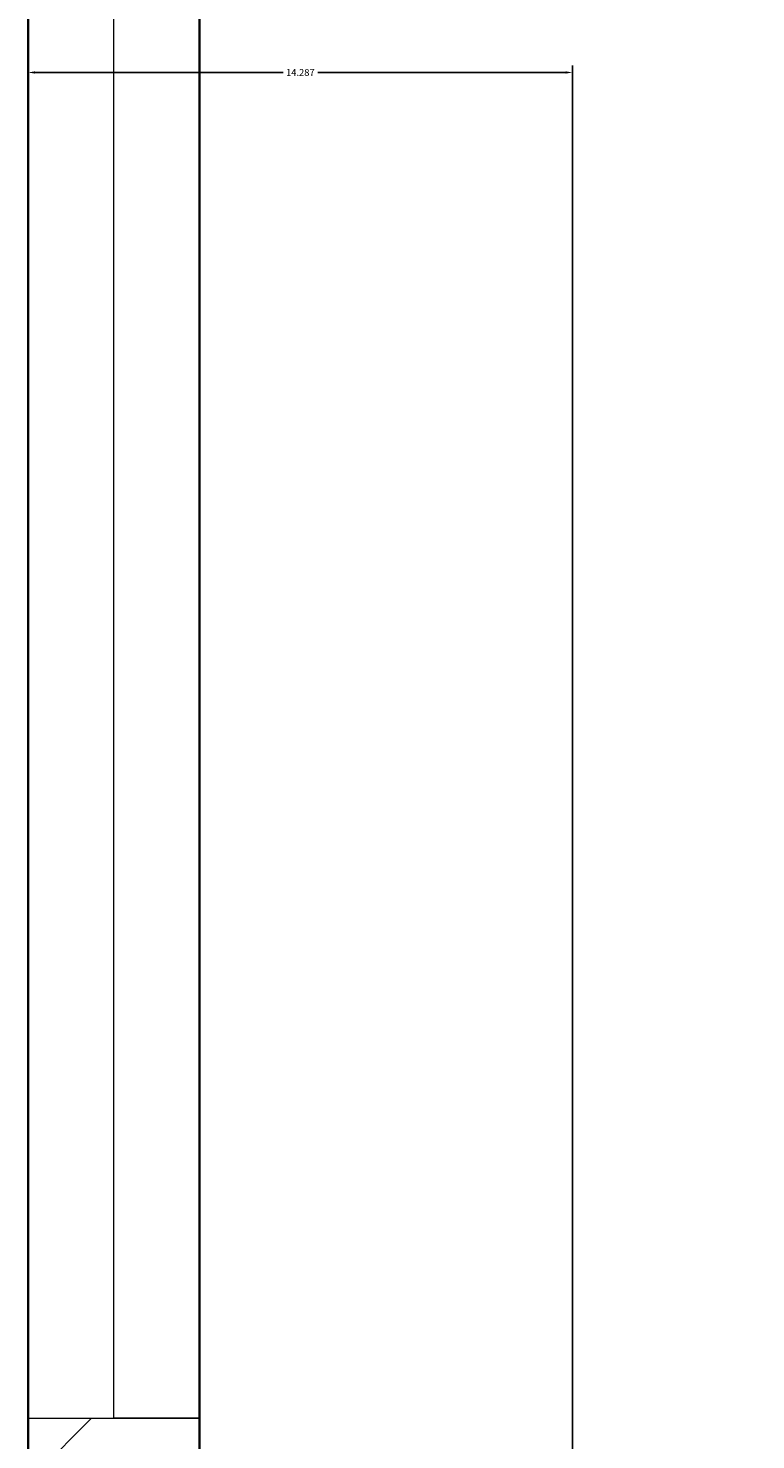
# Model space of a CAD drawing. Units: inches. Extents: x 1962 to 2771, y 1245 to 2660.
# Tile 33 of 114: x 2072 to 2091, y 1952 to 1989. Entities that reach past the tile are written whole.
import ezdxf

# ---------------------------------------------------------------- set-up
doc = ezdxf.new("R2010")
doc.units = ezdxf.units.IN
for name, color, linetype, lineweight in [('A-ANNO-DIMS', 2, 'Continuous', 18), ('A-GLAZ', 4, 'Continuous', 18), ('A-WALL', 7, 'Continuous', 35), ('A-WALL-PATT', 252, 'Continuous', 13)]:
    doc.layers.add(name, color=color, linetype=linetype, lineweight=lineweight)
doc.styles.get("Standard").update_dxf_attribs({"font": 'arial.ttf'})
doc.dimstyles.get("Standard").update_dxf_attribs({"dimtxt": 0.18, "dimasz": 0.18, "dimexe": 0.18, "dimexo": 0.0625, "dimgap": 0.09, "dimtad": 0, "dimtih": 1, "dimtoh": 1, "dimdec": 4, "dimzin": 0, "dimdsep": 46, "dimtxsty": 'Standard', "dimcen": 0.09, "dimadec": 0, "dimazin": 0, "dimtfac": 1, "dimtdec": 4, "dimtofl": 0, "dimtmove": 0, "dimatfit": 3, "dimfxl": 1, "dimtolj": 1, "dimtzin": 0, "dimarcsym": 0})

# ---------------------------------------------------------------- blocks, each defined once
blk = doc.blocks.new('*D41')
at = {"layer": 'A-ANNO-DIMS', "color": 0, "lineweight": -2, "transparency": 16777216}
for p, q in [((2072.02, 1928.906), (2072.02, 1987.974)), ((2086.307, 1928.906), (2086.307, 1987.974)), ((2072.2, 1987.794), (2078.709, 1987.794)), ((2086.127, 1987.794), (2079.619, 1987.794))]:
    blk.add_line(p, q, dxfattribs=at)
at = {"layer": 'A-ANNO-DIMS', "color": 0, "transparency": 16777216}
for points in [[(2072.2, 1987.824), (2072.2, 1987.764), (2072.02, 1987.794)], [(2086.127, 1987.824), (2086.127, 1987.764), (2086.307, 1987.794)]]:
    blk.add_solid(points, dxfattribs=at)
at = {"layer": 'Defpoints', "color": 0, "transparency": 16777216}
for p in [(2086.307, 1987.794), (2072.02, 1928.844), (2086.307, 1928.844)]:
    blk.add_point(p, dxfattribs=at)
at = {"layer": 'A-ANNO-DIMS', "color": 0, "transparency": 16777216, "insert": (2079.164, 1987.794), "char_height": 0.18, "attachment_point": 5}
blk.add_mtext('\\A1;14.287', dxfattribs=at)

msp = doc.modelspace()

# ---------------------------------------------------------------- hatches: boundary and pattern name
at = {"layer": 'A-WALL-PATT'}
h = msp.add_hatch(dxfattribs=at)
h.set_pattern_fill('ANSI32', color=256)
h.paths.add_polyline_path([(2090.8074, 2467.3437), (2141.6481, 2467.3437), (2141.6481, 2469.5937), (2141.6481, 2471.8437), (2086.3074, 2471.8437), (2086.3074, 2422.5333), (2090.8074, 2422.5333)])
h.paths.add_polyline_path([(2282.7664, 2471.8437), (2204.8982, 2471.8437), (2204.8982, 2467.3437), (2234.8074, 2467.3437), (2234.8074, 2311.3437), (2228.7492, 2311.3437), (2228.7492, 2306.8437), (2234.8074, 2306.8437), (2331.9227, 2306.8437), (2331.9227, 2309.0937), (2331.9227, 2311.3437), (2239.3074, 2311.3437), (2239.3074, 2467.3437), (2282.7664, 2467.3437), (2282.7664, 2469.5937)])
h.paths.add_polyline_path([(2471.4531, 2519.8437), (2552.011, 2519.8437), (2564.3996, 2519.8437), (2564.3996, 2511.1389), (2568.8996, 2511.1389), (2568.8996, 2524.3437), (2466.9531, 2524.3437), (2466.9531, 2471.8437), (2450.0749, 2471.8437), (2446.4672, 2471.8437), (2446.4672, 2467.3437), (2450.0749, 2467.3437), (2475.9988, 2467.3437), (2475.9988, 2469.5937), (2475.9988, 2471.8437), (2471.4531, 2471.8437)])
h.paths.add_polyline_path([(2575.2231, 2469.5937), (2575.2231, 2471.8437), (2568.8996, 2471.8437), (2568.8996, 2487.1389), (2564.3996, 2487.1389), (2564.3996, 2471.8437), (2556.511, 2471.8437), (2499.2904, 2471.8437), (2499.2904, 2467.3437), (2507.8074, 2467.3437), (2507.8074, 2311.3437), (2414.863, 2311.3437), (2414.863, 2306.8437), (2512.3074, 2306.8437), (2517.0114, 2306.8437), (2517.0114, 2309.0937), (2517.0114, 2311.3437), (2512.3074, 2311.3437), (2512.3074, 2467.3437), (2575.2231, 2467.3437)])
h.paths.add_polyline_path([(2660.8074, 2471.8437), (2600.9602, 2471.8437), (2600.9602, 2467.3437), (2656.3074, 2467.3437), (2656.3074, 2432.5704), (2660.8074, 2432.5704)])
h.paths.add_polyline_path([(2660.8074, 2372.5704), (2656.3074, 2372.5704), (2656.3074, 2311.3437), (2600.276, 2311.3437), (2600.276, 2309.0937), (2600.276, 2306.8437), (2656.3074, 2306.8437), (2656.3074, 2296.2593), (2660.8074, 2296.2593)])
h.paths.add_polyline_path([(2572.3074, 2306.8437), (2577.1385, 2306.8437), (2577.1385, 2311.3437), (2551.082, 2311.3437), (2551.082, 2306.8437), (2567.8074, 2306.8437), (2567.8074, 2258.8437), (2540.0574, 2258.8437), (2540.0574, 2256.5937), (2540.0574, 2254.3437), (2567.8074, 2254.3437), (2656.3074, 2254.3437), (2656.3074, 2236.9085), (2660.8074, 2236.9085), (2660.8074, 2272.2593), (2656.3074, 2272.2593), (2656.3074, 2258.8437), (2572.3074, 2258.8437)])
h.paths.add_polyline_path([(2512.3074, 2254.3437), (2518.8716, 2254.3437), (2518.8716, 2256.5937), (2518.8716, 2258.8437), (2507.8074, 2258.8437), (2507.8074, 2177.8437), (2567.8074, 2177.8437), (2567.8074, 2172.9628), (2572.3074, 2172.9628), (2572.3074, 2177.8437), (2656.3074, 2177.8437), (2656.3074, 2166.4846), (2660.8074, 2166.4846), (2660.8074, 2200.9085), (2656.3074, 2200.9085), (2656.3074, 2182.3437), (2512.3074, 2182.3437)])
h.paths.add_polyline_path([(2656.3074, 2129.8437), (2572.3074, 2129.8437), (2572.3074, 2150.3044), (2570.0574, 2150.3044), (2567.8074, 2150.3044), (2567.8074, 2129.8437), (2507.8074, 2129.8437), (2507.8074, 2116.3027), (2510.0574, 2116.3027), (2512.3074, 2116.3027), (2512.3074, 2125.3437), (2567.8074, 2125.3437), (2572.3074, 2125.3437), (2656.3074, 2125.3437)])
h.paths.add_polyline_path([(2090.8074, 2362.5333), (2086.3074, 2362.5333), (2086.3074, 2298.6242), (2090.8074, 2298.6242), (2090.8074, 2306.8437), (2174.8074, 2306.8437), (2174.8074, 2286.4178), (2179.3074, 2286.4178), (2179.3074, 2306.8437), (2192.8641, 2306.8437), (2192.8641, 2309.0937), (2192.8641, 2311.3437), (2090.8074, 2311.3437)])
h.paths.add_polyline_path([(2209.156, 2258.8437), (2179.3074, 2258.8437), (2179.3074, 2263.2236), (2177.0574, 2263.2236), (2174.8074, 2263.2236), (2174.8074, 2258.8437), (2090.8074, 2258.8437), (2090.8074, 2274.6242), (2086.3074, 2274.6242), (2086.3074, 2238.2967), (2088.5574, 2238.2967), (2090.8074, 2238.2967), (2090.8074, 2254.3437), (2209.156, 2254.3437)])
h.paths.add_polyline_path([(2090.8074, 2177.8437), (2234.8074, 2177.8437), (2234.8074, 2173.1428), (2239.3074, 2173.1428), (2239.3074, 2258.8437), (2230.8442, 2258.8437), (2230.8442, 2256.5937), (2230.8442, 2254.3437), (2234.8074, 2254.3437), (2234.8074, 2182.3437), (2090.8074, 2182.3437), (2090.8074, 2202.2967), (2086.3074, 2202.2967), (2086.3074, 2140.0389), (2090.8074, 2140.0389)])
h.paths.add_polyline_path([(2090.8074, 2080.0389), (2086.3074, 2080.0389), (2086.3074, 2033.8437), (2090.8074, 2033.8437)], flags=17)
h.paths.add_polyline_path([(2244.9405, 2033.8437), (2239.3074, 2033.8437), (2239.3074, 2142.0665), (2237.2592, 2142.0665), (2234.8074, 2142.0665), (2234.8074, 2033.8437), (2090.8074, 2033.8437), (2076.5204, 2033.8437), (2072.0204, 2033.8437), (2072.0204, 2000.4493), (2076.5204, 2000.4493), (2076.5204, 2029.3437), (2090.8074, 2029.3437), (2244.9405, 2029.3437), (2244.9405, 2031.5937)])
h.paths.add_polyline_path([(2234.8074, 1933.3437), (2076.5204, 1933.3437), (2076.5204, 1952.4493), (2074.2704, 1952.4493), (2072.0204, 1952.4493), (2072.0204, 1933.3437), (2072.0204, 1928.8437), (2234.8074, 1928.8437)])
h.paths.add_polyline_path([(2090.8074, 1928.8437), (2086.3074, 1928.8437), (2086.3074, 1906.5013), (2090.8074, 1906.5013)])
h.paths.add_polyline_path([(2090.8074, 1846.5013), (2086.3074, 1846.5013), (2086.3074, 1769.9917), (2088.5574, 1769.9917), (2090.8074, 1769.9917), (2090.8074, 1780.3437), (2234.8074, 1780.3437), (2234.8074, 1708.3437), (2230.3764, 1708.3437), (2230.3764, 1703.8437), (2239.3074, 1703.8437), (2239.3074, 1792.6669), (2237.0574, 1792.6669), (2234.8074, 1792.6669), (2234.8074, 1784.8437), (2090.8074, 1784.8437)])
h.paths.add_polyline_path([(2239.3074, 1928.8437), (2244.9405, 1928.8437), (2244.9405, 1931.0937), (2244.9405, 1933.3437), (2234.8074, 1933.3437), (2234.8074, 1928.8437), (2234.8074, 1825.5949), (2239.3074, 1825.5949)])
h.paths.add_polyline_path([(2148.0425, 1649.0937), (2148.0425, 1651.3437), (2090.8074, 1651.3437), (2090.8074, 1646.8437), (2148.0425, 1646.8437)], flags=0)
h.paths.add_polyline_path([(2207.5601, 1708.3437), (2090.8074, 1708.3437), (2090.8074, 1703.8437), (2174.8074, 1703.8437), (2174.8074, 1651.3437), (2170.4457, 1651.3437), (2170.4457, 1646.8437), (2195.9924, 1646.8437), (2195.9924, 1649.0937), (2195.9924, 1651.3437), (2179.3074, 1651.3437), (2179.3074, 1703.8437), (2207.5601, 1703.8437), (2207.5601, 1706.0937)])
h.paths.add_polyline_path([(2090.8074, 1733.9917), (2086.3074, 1733.9917), (2086.3074, 1696.1032), (2088.5574, 1696.1032), (2090.8074, 1696.1032)])
h.paths.add_polyline_path([(2090.8074, 1672.1032), (2086.3074, 1672.1032), (2086.3074, 1600.3335), (2090.8074, 1600.3335)])
h.paths.add_polyline_path([(2090.8074, 1540.3335), (2086.3074, 1540.3335), (2086.3074, 1486.3437), (2139.6766, 1486.3437), (2139.6766, 1490.8437), (2090.8074, 1490.8437)])
h.paths.add_polyline_path([(2302.3876, 1490.8437), (2239.3074, 1490.8437), (2239.3074, 1646.8437), (2335.9994, 1646.8437), (2335.9994, 1651.3437), (2229.884, 1651.3437), (2229.884, 1646.8437), (2234.8074, 1646.8437), (2234.8074, 1490.8437), (2202.7103, 1490.8437), (2202.7103, 1488.5937), (2202.7103, 1486.3437), (2275.0699, 1486.3437), (2275.0699, 1475.772), (2279.5699, 1475.772), (2279.5699, 1486.3437), (2302.3876, 1486.3437)])
h.paths.add_polyline_path([(2279.5699, 1451.772), (2275.0699, 1451.772), (2275.0699, 1438.3437), (2174.8074, 1438.3437), (2174.8074, 1486.3437), (2179.7922, 1486.3437), (2179.7922, 1490.8437), (2163.3585, 1490.8437), (2163.3585, 1488.5937), (2163.3585, 1486.3437), (2170.3074, 1486.3437), (2170.3074, 1433.8437), (2279.5699, 1433.8437)])
h.paths.add_polyline_path([(2427.2363, 1490.8437), (2375.8074, 1490.8437), (2375.8074, 1646.8437), (2381.6401, 1646.8437), (2381.6401, 1651.3437), (2365.887, 1651.3437), (2365.887, 1649.0937), (2365.887, 1646.8437), (2371.3074, 1646.8437), (2371.3074, 1490.8437), (2327.5627, 1490.8437), (2327.5627, 1488.5937), (2327.5627, 1486.3437), (2371.3074, 1486.3437), (2371.3074, 1433.8437), (2375.8074, 1433.8437), (2375.8074, 1486.3437), (2427.2363, 1486.3437)])
h.paths.add_polyline_path([(2512.3074, 1646.8437), (2519.4351, 1646.8437), (2519.4351, 1649.0937), (2519.4351, 1651.3437), (2507.8074, 1651.3437), (2416.0063, 1651.3437), (2416.0063, 1649.0937), (2416.0063, 1646.8437), (2507.8074, 1646.8437), (2507.8074, 1490.8437), (2497.0532, 1490.8437), (2497.0532, 1488.5937), (2497.0532, 1486.3437), (2574.9344, 1486.3437), (2574.9344, 1476.0181), (2579.4344, 1476.0181), (2579.4344, 1486.3437), (2584.4872, 1486.3437), (2584.3074, 1490.8437), (2512.3074, 1490.8437)])
h.paths.add_polyline_path([(2470.5091, 1486.3437), (2473.9767, 1486.3437), (2473.9767, 1490.8437), (2449.6605, 1490.8437), (2449.6605, 1488.5937), (2449.6605, 1486.3437), (2466.0091, 1486.3437), (2466.0091, 1433.8437), (2470.5091, 1433.8437), (2579.4344, 1433.8437), (2579.4344, 1452.0181), (2574.9344, 1452.0181), (2574.9344, 1438.3437), (2554.5091, 1438.3437), (2470.5091, 1438.3437)])
h.paths.add_polyline_path([(2656.3074, 1490.8437), (2611.86, 1490.8437), (2611.86, 1486.3437), (2656.3074, 1486.3437)])
h.paths.add_polyline_path([(2660.8074, 1532.7007), (2658.5574, 1532.7007), (2656.3074, 1532.7007), (2656.3074, 1486.3437), (2660.8074, 1486.3437)])
h.paths.add_polyline_path([(2660.8074, 1664.9663), (2656.3074, 1664.9663), (2656.3074, 1651.3437), (2602.2313, 1651.3437), (2602.2313, 1646.8437), (2656.3074, 1646.8437), (2656.3074, 1592.7007), (2660.8074, 1592.7007)])
h.paths.add_polyline_path([(2660.8074, 1724.5221), (2656.3074, 1724.5221), (2656.3074, 1703.8437), (2542.4725, 1703.8437), (2542.4725, 1699.3437), (2567.8074, 1699.3437), (2567.8074, 1651.3437), (2552.7766, 1651.3437), (2552.7766, 1649.0937), (2552.7766, 1646.8437), (2577.2878, 1646.8437), (2577.2878, 1649.0937), (2577.2878, 1651.3437), (2572.3074, 1651.3437), (2572.3074, 1699.3437), (2656.3074, 1699.3437), (2656.3074, 1688.9663), (2660.8074, 1688.9663)])
h.paths.add_polyline_path([(2660.8074, 1880.6524), (2656.3074, 1880.6524), (2656.3074, 1832.8437), (2512.3074, 1832.8437), (2512.3074, 1837.8959), (2507.8074, 1837.8959), (2507.8074, 1828.3437), (2567.8074, 1828.3437), (2567.8074, 1804.3437), (2572.3074, 1804.3437), (2572.3074, 1828.3437), (2656.3074, 1828.3437), (2656.3074, 1818.6778), (2660.8074, 1818.6778)])
h.paths.add_polyline_path([(2660.8074, 1794.6778), (2656.3074, 1794.6778), (2656.3074, 1780.3437), (2572.3074, 1780.3437), (2572.3074, 1783.0303), (2570.0574, 1783.0303), (2567.8074, 1783.0303), (2567.8074, 1780.3437), (2507.8074, 1780.3437), (2507.8074, 1699.3437), (2517.8858, 1699.3437), (2517.8858, 1701.5937), (2517.8858, 1703.8437), (2512.3074, 1703.8437), (2512.3074, 1775.8437), (2656.3074, 1775.8437), (2656.3074, 1760.5221), (2660.8074, 1760.5221)])
h.paths.add_polyline_path([(2660.8074, 1981.3437), (2660.8074, 2020.2808), (2658.5574, 2020.2808), (2656.3074, 2020.2808), (2656.3074, 1981.3437), (2512.3074, 1981.3437), (2512.3074, 2086.6996), (2507.8074, 2086.6996), (2507.8074, 1981.3437), (2375.8074, 1981.3437), (2375.8074, 1986.8505), (2373.5574, 1986.8505), (2371.3074, 1986.8505), (2371.3074, 1973.2607), (2375.8074, 1973.2607), (2375.8074, 1976.8437), (2507.8074, 1976.8437), (2507.8074, 1865.4281), (2510.0574, 1865.4281), (2512.3074, 1865.4281), (2512.3074, 1976.8437), (2660.8074, 1976.8437)])
h.paths.add_polyline_path([(2375.8074, 1940.297), (2373.5574, 1940.297), (2371.3074, 1940.297), (2371.3074, 1933.3437), (2278.4434, 1933.3437), (2278.4434, 1928.8437), (2371.3074, 1928.8437), (2371.3074, 1651.3437), (2375.8074, 1651.3437)])
h.paths.add_polyline_path([(2660.8074, 1976.8437), (2656.3074, 1976.8437), (2656.3074, 1940.6524), (2660.8074, 1940.6524)], flags=17)
h.paths.add_polyline_path([(2660.8074, 2142.4846), (2656.3074, 2142.4846), (2656.3074, 2080.2808), (2660.8074, 2080.2808)])
h.paths.add_polyline_path([(2381.4189, 2311.3437), (2375.8074, 2311.3437), (2375.8074, 2467.3437), (2424.7242, 2467.3437), (2424.7242, 2469.5937), (2424.7242, 2471.8437), (2375.8074, 2471.8437), (2375.8074, 2524.3437), (2371.3074, 2524.3437), (2371.3074, 2471.8437), (2307.2097, 2471.8437), (2307.2097, 2467.3437), (2371.3074, 2467.3437), (2371.3074, 2311.3437), (2366.8901, 2311.3437), (2366.8901, 2306.8437), (2371.3074, 2306.8437), (2371.3074, 2033.8437), (2279.6589, 2033.8437), (2279.6589, 2029.3437), (2371.3074, 2029.3437), (2371.3074, 2014.2598), (2375.8074, 2014.2598), (2375.8074, 2306.8437), (2381.4189, 2306.8437)])
h.paths.add_polyline_path([(2263.3074, 2524.3437), (2170.3074, 2524.3437), (2170.3074, 2519.8437), (2170.3074, 2471.8437), (2165.0312, 2471.8437), (2165.0312, 2467.3437), (2179.6721, 2467.3437), (2179.6721, 2469.5161), (2179.6721, 2471.8437), (2174.8074, 2471.8437), (2174.8074, 2519.8437), (2258.8074, 2519.8437), (2258.8074, 2511.6436), (2263.3074, 2511.6436)])
h.paths.add_polyline_path([(2245.0232, 1361.4123), (2492.9468, 1361.4123), (2492.9468, 1398.505), (2245.0232, 1398.505)], flags=9)
h.paths.add_polyline_path([(2388.1434, 2086.6936), (2425.0704, 2086.6936), (2425.0704, 2105.3509), (2388.1434, 2105.3509)], flags=9)
h.paths.add_polyline_path([(2404.922, 2242.6744), (2445.7337, 2242.6744), (2445.7337, 2261.3318), (2404.922, 2261.3318)], flags=9)
h.paths.add_polyline_path([(2269.4107, 2156.7935), (2306.3378, 2156.7935), (2306.3378, 2175.4508), (2269.4107, 2175.4508)], flags=9)
h.paths.add_polyline_path([(2269.3277, 2233.4343), (2306.2547, 2233.4343), (2306.2547, 2252.0917), (2269.3277, 2252.0917)], flags=9)
h.paths.add_polyline_path([(2431.6052, 2320.6922), (2470.4456, 2320.6922), (2470.4456, 2339.3495), (2431.6052, 2339.3495)], flags=25)
h.paths.add_polyline_path([(2249.6902, 2315.7608), (2288.5306, 2315.7608), (2288.5306, 2334.4182), (2249.6902, 2334.4182)], flags=25)
h.paths.add_polyline_path([(2096.9301, 2314.3181), (2135.7704, 2314.3181), (2135.7704, 2332.9755), (2096.9301, 2332.9755)], flags=25)
h.paths.add_polyline_path([(2134.3475, 2285.7089), (2161.4655, 2285.7089), (2161.4655, 2304.3662), (2134.3475, 2304.3662)], flags=9)
h.paths.add_polyline_path([(2126.5155, 2209.4076), (2159.9227, 2209.4076), (2159.9227, 2228.065), (2126.5155, 2228.065)], flags=25)
h.paths.add_polyline_path([(2110.5753, 2141.5299), (2149.4157, 2141.5299), (2149.4157, 2160.1872), (2110.5753, 2160.1872)], flags=25)
h.paths.add_polyline_path([(2249.8618, 1968.3317), (2286.3966, 1968.3317), (2286.3966, 1986.989), (2249.8618, 1986.989)], flags=9)
h.paths.add_polyline_path([(2395.9507, 1777.0051), (2436.7624, 1777.0051), (2436.7624, 1795.6625), (2395.9507, 1795.6625)], flags=9)
h.paths.add_polyline_path([(2398.5259, 1888.5651), (2435.0062, 1888.5651), (2435.0062, 1907.2224), (2398.5259, 1907.2224)], flags=25)
h.paths.add_polyline_path([(2259.3506, 1728.3559), (2296.2776, 1728.3559), (2296.2776, 1747.0132), (2259.3506, 1747.0132)], flags=9)
h.paths.add_polyline_path([(2271.3698, 1845.268), (2308.2968, 1845.268), (2308.2968, 1863.9253), (2271.3698, 1863.9253)], flags=9)
h.paths.add_polyline_path([(2120.9355, 1786.3027), (2159.7759, 1786.3027), (2159.7759, 1804.9601), (2120.9355, 1804.9601)], flags=25)
h.paths.add_polyline_path([(2121.3164, 1732.1043), (2154.7236, 1732.1043), (2154.7236, 1750.7616), (2121.3164, 1750.7616)], flags=25)
h.paths.add_polyline_path([(2118.3706, 1678.8997), (2147.5282, 1678.8997), (2147.5282, 1697.557), (2118.3706, 1697.557)], flags=25)
h.paths.add_polyline_path([(2385.9227, 1493.557), (2424.763, 1493.557), (2424.763, 1512.2143), (2385.9227, 1512.2143)], flags=25)
h.paths.add_polyline_path([(2248.7058, 1500.0256), (2287.5462, 1500.0256), (2287.5462, 1518.6829), (2248.7058, 1518.6829)], flags=25)
h.paths.add_polyline_path([(2104.1669, 1617.3771), (2143.0073, 1617.3771), (2143.0073, 1636.0344), (2104.1669, 1636.0344)], flags=9)
h.paths.add_polyline_path([(2096.0714, 1447.8824), (2137.3845, 1447.8824), (2137.3845, 1458.1859), (2096.0714, 1458.1859)], flags=9)
h.paths.add_polyline_path([(2180.6114, 1440.325), (2209.7689, 1440.325), (2209.7689, 1458.9823), (2180.6114, 1458.9823)], flags=25)
h.paths.add_polyline_path([(2316.1698, 1447.9637), (2357.4829, 1447.9637), (2357.4829, 1458.2673), (2316.1698, 1458.2673)], flags=9)
h.paths.add_polyline_path([(2397.6187, 1447.9637), (2438.9318, 1447.9637), (2438.9318, 1458.2673), (2397.6187, 1458.2673)], flags=9)
h.paths.add_polyline_path([(2473.0778, 1439.5953), (2502.2354, 1439.5953), (2502.2354, 1458.2527), (2473.0778, 1458.2527)], flags=25)
h.paths.add_polyline_path([(2589.7027, 1447.8819), (2631.0158, 1447.8819), (2631.0158, 1458.1855), (2589.7027, 1458.1855)], flags=9)
h.paths.add_polyline_path([(2522.4009, 1497.5285), (2561.2413, 1497.5285), (2561.2413, 1516.1859), (2522.4009, 1516.1859)], flags=25)
h.paths.add_polyline_path([(2579.6565, 1671.3482), (2608.8141, 1671.3482), (2608.8141, 1690.0056), (2579.6565, 1690.0056)], flags=25)
h.paths.add_polyline_path([(2544.7038, 1725.5064), (2578.1111, 1725.5064), (2578.1111, 1744.1637), (2544.7038, 1744.1637)], flags=25)
h.paths.add_polyline_path([(2578.1191, 1807.472), (2607.2766, 1807.472), (2607.2766, 1826.1293), (2578.1191, 1826.1293)], flags=25)
h.paths.add_polyline_path([(2595.0614, 1835.1839), (2633.9018, 1835.1839), (2633.9018, 1853.8413), (2595.0614, 1853.8413)], flags=25)
h.paths.add_polyline_path([(2567.0097, 2097.7035), (2605.8501, 2097.7035), (2605.8501, 2116.3609), (2567.0097, 2116.3609)], flags=9)
h.paths.add_polyline_path([(2586.644, 2134.6454), (2615.8015, 2134.6454), (2615.8015, 2153.3027), (2586.644, 2153.3027)], flags=9)
h.paths.add_polyline_path([(2544.6185, 2212.6783), (2578.0258, 2212.6783), (2578.0258, 2231.3356), (2544.6185, 2231.3356)], flags=25)
h.paths.add_polyline_path([(2577.0273, 2256.9023), (2606.1849, 2256.9023), (2606.1849, 2275.5597), (2577.0273, 2275.5597)], flags=24)
h.paths.add_polyline_path([(2605.2683, 2315.2821), (2644.1087, 2315.2821), (2644.1087, 2333.9395), (2605.2683, 2333.9395)], flags=25)
h.paths.add_polyline_path([(2583.1244, 2496.1815), (2624.4375, 2496.1815), (2624.4375, 2506.4851), (2583.1244, 2506.4851)], flags=9)
h.paths.add_polyline_path([(2474.761, 2497.0823), (2503.9185, 2497.0823), (2503.9185, 2515.7397), (2474.761, 2515.7397)], flags=25)
h.paths.add_polyline_path([(2387.5787, 2494.2563), (2428.902, 2494.2563), (2428.902, 2504.5598), (2387.5787, 2504.5598)], flags=9)
h.paths.add_polyline_path([(2300.1657, 2500.1564), (2341.4788, 2500.1564), (2341.4788, 2510.46), (2300.1657, 2510.46)], flags=25)
h.paths.add_polyline_path([(2176.8589, 2497.5843), (2206.0165, 2497.5843), (2206.0165, 2516.2416), (2176.8589, 2516.2416)], flags=25)
h.paths.add_polyline_path([(2097.4668, 2494.9762), (2138.7799, 2494.9762), (2138.7799, 2505.2798), (2097.4668, 2505.2798)], flags=9)

# ---------------------------------------------------------------- linework, layer by layer
at = {"layer": 'A-GLAZ'}
for p, q in [((2074.2704, 1952.4493), (2074.2704, 2000.4493)), ((2072.0204, 1952.4493), (2076.5204, 1952.4493)), ((2076.5204, 1952.4493), (2074.2704, 1952.4493))]:
    msp.add_line(p, q, dxfattribs=at)
at = {"layer": 'A-WALL'}
for p, q in [((2072.0204, 2033.8437), (2072.0204, 1933.3437)), ((2076.5204, 2029.3437), (2076.5204, 1933.3437))]:
    msp.add_line(p, q, dxfattribs=at)

# ---------------------------------------------------------------- dimensions: what is measured, and where the dimension line sits
at = {"layer": 'A-ANNO-DIMS'}
dim = msp.add_linear_dim(base=(2086.3074, 1987.7937), p1=(2072.0204, 1928.8437), p2=(2086.3074, 1928.8437), dimstyle='Standard', override={"dimdec": 3, "dimlfac": 1, "dimrnd": 0, "dimzin": 0, "dimdsep": 46, "dimlunit": 2}, dxfattribs=at)
dim.commit()
dim.dimension.update_dxf_attribs({"geometry": '*D41', "text_midpoint": (2079.1639, 1987.7937)})

doc.saveas('drawing.dxf')
